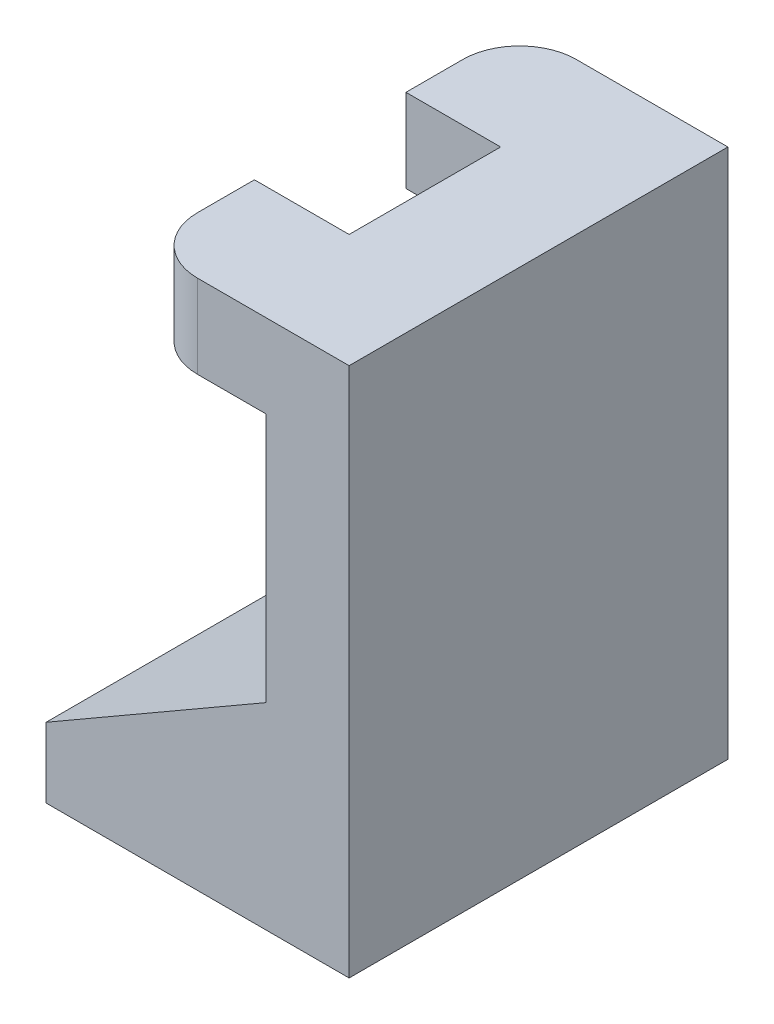
ISO-10303-21;
HEADER;
FILE_DESCRIPTION(('STEP AP214'),'2;1');
FILE_NAME('part.step','',(''),(''),'','','');
FILE_SCHEMA(('AUTOMOTIVE_DESIGN { 1 0 10303 214 1 1 1 1 }'));
ENDSEC;
DATA;
#1=APPLICATION_CONTEXT('core data for automotive mechanical design processes');
#2=APPLICATION_PROTOCOL_DEFINITION('international standard','automotive_design',2000,#1);
#3=PRODUCT_CONTEXT('',#1,'mechanical');
#4=PRODUCT('Part','Part','',(#3));
#5=PRODUCT_RELATED_PRODUCT_CATEGORY('part','',(#4));
#6=PRODUCT_DEFINITION_FORMATION('','',#4);
#7=PRODUCT_DEFINITION_CONTEXT('part definition',#1,'design');
#8=PRODUCT_DEFINITION('design','',#6,#7);
#9=PRODUCT_DEFINITION_SHAPE('','',#8);
#10=(LENGTH_UNIT() NAMED_UNIT(*) SI_UNIT(.MILLI.,.METRE.));
#11=(NAMED_UNIT(*) PLANE_ANGLE_UNIT() SI_UNIT($,.RADIAN.));
#12=(NAMED_UNIT(*) SI_UNIT($,.STERADIAN.) SOLID_ANGLE_UNIT());
#13=UNCERTAINTY_MEASURE_WITH_UNIT(LENGTH_MEASURE(1.E-05),#10,'distance_accuracy_value','');
#14=(GEOMETRIC_REPRESENTATION_CONTEXT(3) GLOBAL_UNCERTAINTY_ASSIGNED_CONTEXT((#13)) GLOBAL_UNIT_ASSIGNED_CONTEXT((#10,
#11,#12)) REPRESENTATION_CONTEXT('',''));
#15=CARTESIAN_POINT('',(0.,0.,0.));
#16=DIRECTION('',(0.,0.,1.));
#17=DIRECTION('',(1.,0.,0.));
#18=AXIS2_PLACEMENT_3D('',#15,#16,#17);
#19=CARTESIAN_POINT('',(0.5,2.8,-2.));
#20=DIRECTION('',(-1.,0.,0.));
#21=DIRECTION('',(0.,-1.,0.));
#22=AXIS2_PLACEMENT_3D('',#19,#20,#21);
#23=PLANE('',#22);
#24=DIRECTION('',(0.,1.,0.));
#25=VECTOR('',#24,1.);
#26=CARTESIAN_POINT('',(0.5,2.36,-0.6));
#27=LINE('',#26,#25);
#28=CARTESIAN_POINT('',(0.5,2.36,-0.6));
#29=VERTEX_POINT('',#28);
#30=CARTESIAN_POINT('',(0.5,2.8,-0.6));
#31=VERTEX_POINT('',#30);
#32=EDGE_CURVE('E181',#29,#31,#27,.T.);
#33=ORIENTED_EDGE('',*,*,#32,.F.);
#34=DIRECTION('',(0.,0.,1.));
#35=VECTOR('',#34,1.);
#36=CARTESIAN_POINT('',(0.5,2.36,-2.));
#37=LINE('',#36,#35);
#38=CARTESIAN_POINT('',(0.5,2.36,-0.3));
#39=VERTEX_POINT('',#38);
#40=EDGE_CURVE('E246',#29,#39,#37,.T.);
#41=ORIENTED_EDGE('',*,*,#40,.T.);
#42=DIRECTION('',(0.,1.,0.));
#43=VECTOR('',#42,1.);
#44=CARTESIAN_POINT('',(0.5,2.36,-0.3));
#45=LINE('',#44,#43);
#46=CARTESIAN_POINT('',(0.5,2.8,-0.3));
#47=VERTEX_POINT('',#46);
#48=EDGE_CURVE('E192',#39,#47,#45,.T.);
#49=ORIENTED_EDGE('',*,*,#48,.T.);
#50=DIRECTION('',(0.,0.,1.));
#51=VECTOR('',#50,1.);
#52=CARTESIAN_POINT('',(0.5,2.8,-2.));
#53=LINE('',#52,#51);
#54=EDGE_CURVE('E255',#31,#47,#53,.T.);
#55=ORIENTED_EDGE('',*,*,#54,.F.);
#56=EDGE_LOOP('',(#33,#41,#49,#55));
#57=FACE_BOUND('',#56,.T.);
#58=ADVANCED_FACE('F44',(#57),#23,.T.);
#59=DIRECTION('',(0.,1.,0.));
#60=VECTOR('',#59,1.);
#61=CARTESIAN_POINT('',(0.5,2.36,-1.4));
#62=LINE('',#61,#60);
#63=CARTESIAN_POINT('',(0.5,2.36,-1.4));
#64=VERTEX_POINT('',#63);
#65=CARTESIAN_POINT('',(0.5,2.8,-1.4));
#66=VERTEX_POINT('',#65);
#67=EDGE_CURVE('E160',#64,#66,#62,.T.);
#68=ORIENTED_EDGE('',*,*,#67,.T.);
#69=CARTESIAN_POINT('',(0.5,2.8,-1.7));
#70=VERTEX_POINT('',#69);
#71=EDGE_CURVE('E253',#70,#66,#53,.T.);
#72=ORIENTED_EDGE('',*,*,#71,.F.);
#73=DIRECTION('',(0.,1.,0.));
#74=VECTOR('',#73,1.);
#75=CARTESIAN_POINT('',(0.5,2.36,-1.7));
#76=LINE('',#75,#74);
#77=CARTESIAN_POINT('',(0.5,2.36,-1.7));
#78=VERTEX_POINT('',#77);
#79=EDGE_CURVE('E189',#78,#70,#76,.T.);
#80=ORIENTED_EDGE('',*,*,#79,.F.);
#81=EDGE_CURVE('E248',#78,#64,#37,.T.);
#82=ORIENTED_EDGE('',*,*,#81,.T.);
#83=EDGE_LOOP('',(#68,#72,#80,#82));
#84=FACE_BOUND('',#83,.T.);
#85=ADVANCED_FACE('F296',(#84),#23,.T.);
#86=CARTESIAN_POINT('',(0.,0.,-2.));
#87=DIRECTION('',(0.,0.,1.));
#88=DIRECTION('',(1.,0.,0.));
#89=AXIS2_PLACEMENT_3D('',#86,#87,#88);
#90=PLANE('',#89);
#91=DIRECTION('',(0.,1.,0.));
#92=VECTOR('',#91,1.);
#93=CARTESIAN_POINT('',(0.8,2.36,-2.));
#94=LINE('',#93,#92);
#95=CARTESIAN_POINT('',(0.8,2.36,-2.));
#96=VERTEX_POINT('',#95);
#97=CARTESIAN_POINT('',(0.8,2.8,-2.));
#98=VERTEX_POINT('',#97);
#99=EDGE_CURVE('E195',#96,#98,#94,.T.);
#100=ORIENTED_EDGE('',*,*,#99,.T.);
#101=DIRECTION('',(-1.,0.,0.));
#102=VECTOR('',#101,1.);
#103=CARTESIAN_POINT('',(1.6,2.8,-2.));
#104=LINE('',#103,#102);
#105=CARTESIAN_POINT('',(1.6,2.8,-2.));
#106=VERTEX_POINT('',#105);
#107=EDGE_CURVE('E214',#106,#98,#104,.T.);
#108=ORIENTED_EDGE('',*,*,#107,.F.);
#109=DIRECTION('',(0.,1.,0.));
#110=VECTOR('',#109,1.);
#111=CARTESIAN_POINT('',(1.6,0.,-2.));
#112=LINE('',#111,#110);
#113=CARTESIAN_POINT('',(1.6,0.,-2.));
#114=VERTEX_POINT('',#113);
#115=EDGE_CURVE('E215',#114,#106,#112,.T.);
#116=ORIENTED_EDGE('',*,*,#115,.F.);
#117=DIRECTION('',(1.,0.,0.));
#118=VECTOR('',#117,1.);
#119=CARTESIAN_POINT('',(0.,0.,-2.));
#120=LINE('',#119,#118);
#121=CARTESIAN_POINT('',(0.,0.,-2.));
#122=VERTEX_POINT('',#121);
#123=EDGE_CURVE('E208',#122,#114,#120,.T.);
#124=ORIENTED_EDGE('',*,*,#123,.F.);
#125=DIRECTION('',(0.,-1.,0.));
#126=VECTOR('',#125,1.);
#127=CARTESIAN_POINT('',(0.,0.,-2.));
#128=LINE('',#127,#126);
#129=CARTESIAN_POINT('',(0.,0.369422221254713,-2.));
#130=VERTEX_POINT('',#129);
#131=EDGE_CURVE('E202',#130,#122,#128,.T.);
#132=ORIENTED_EDGE('',*,*,#131,.F.);
#133=DIRECTION('',(-0.866025403784438,-0.500000000000001,0.));
#134=VECTOR('',#133,1.);
#135=CARTESIAN_POINT('',(0.,0.369422221254713,-2.));
#136=LINE('',#135,#134);
#137=CARTESIAN_POINT('',(1.16,1.03914853351468,-2.));
#138=VERTEX_POINT('',#137);
#139=EDGE_CURVE('E224',#138,#130,#136,.T.);
#140=ORIENTED_EDGE('',*,*,#139,.F.);
#141=DIRECTION('',(0.,-1.,0.));
#142=VECTOR('',#141,1.);
#143=CARTESIAN_POINT('',(1.16,2.36,-2.));
#144=LINE('',#143,#142);
#145=CARTESIAN_POINT('',(1.16,2.36,-2.));
#146=VERTEX_POINT('',#145);
#147=EDGE_CURVE('E219',#146,#138,#144,.T.);
#148=ORIENTED_EDGE('',*,*,#147,.F.);
#149=DIRECTION('',(1.,0.,0.));
#150=VECTOR('',#149,1.);
#151=CARTESIAN_POINT('',(1.16,2.36,-2.));
#152=LINE('',#151,#150);
#153=EDGE_CURVE('E217',#96,#146,#152,.T.);
#154=ORIENTED_EDGE('',*,*,#153,.F.);
#155=EDGE_LOOP('',(#100,#108,#116,#124,#132,#140,#148,#154));
#156=FACE_BOUND('',#155,.T.);
#157=ADVANCED_FACE('F272',(#156),#90,.F.);
#158=CARTESIAN_POINT('',(0.,0.,0.));
#159=DIRECTION('',(0.,0.,1.));
#160=DIRECTION('',(1.,0.,0.));
#161=AXIS2_PLACEMENT_3D('',#158,#159,#160);
#162=PLANE('',#161);
#163=DIRECTION('',(-1.,0.,0.));
#164=VECTOR('',#163,1.);
#165=CARTESIAN_POINT('',(1.6,2.8,0.));
#166=LINE('',#165,#164);
#167=CARTESIAN_POINT('',(1.6,2.8,0.));
#168=VERTEX_POINT('',#167);
#169=CARTESIAN_POINT('',(0.8,2.8,0.));
#170=VERTEX_POINT('',#169);
#171=EDGE_CURVE('E234',#168,#170,#166,.T.);
#172=ORIENTED_EDGE('',*,*,#171,.T.);
#173=DIRECTION('',(0.,1.,0.));
#174=VECTOR('',#173,1.);
#175=CARTESIAN_POINT('',(0.8,2.36,0.));
#176=LINE('',#175,#174);
#177=CARTESIAN_POINT('',(0.8,2.36,0.));
#178=VERTEX_POINT('',#177);
#179=EDGE_CURVE('E200',#178,#170,#176,.T.);
#180=ORIENTED_EDGE('',*,*,#179,.F.);
#181=DIRECTION('',(1.,0.,0.));
#182=VECTOR('',#181,1.);
#183=CARTESIAN_POINT('',(1.16,2.36,0.));
#184=LINE('',#183,#182);
#185=CARTESIAN_POINT('',(1.16,2.36,0.));
#186=VERTEX_POINT('',#185);
#187=EDGE_CURVE('E240',#178,#186,#184,.T.);
#188=ORIENTED_EDGE('',*,*,#187,.T.);
#189=DIRECTION('',(0.,-1.,0.));
#190=VECTOR('',#189,1.);
#191=CARTESIAN_POINT('',(1.16,2.36,0.));
#192=LINE('',#191,#190);
#193=CARTESIAN_POINT('',(1.16,1.03914853351468,0.));
#194=VERTEX_POINT('',#193);
#195=EDGE_CURVE('E239',#186,#194,#192,.T.);
#196=ORIENTED_EDGE('',*,*,#195,.T.);
#197=DIRECTION('',(-0.866025403784438,-0.500000000000001,0.));
#198=VECTOR('',#197,1.);
#199=CARTESIAN_POINT('',(0.,0.369422221254713,0.));
#200=LINE('',#199,#198);
#201=CARTESIAN_POINT('',(0.,0.369422221254713,0.));
#202=VERTEX_POINT('',#201);
#203=EDGE_CURVE('E207',#194,#202,#200,.T.);
#204=ORIENTED_EDGE('',*,*,#203,.T.);
#205=DIRECTION('',(0.,-1.,0.));
#206=VECTOR('',#205,1.);
#207=CARTESIAN_POINT('',(0.,0.,0.));
#208=LINE('',#207,#206);
#209=CARTESIAN_POINT('',(0.,0.,0.));
#210=VERTEX_POINT('',#209);
#211=EDGE_CURVE('E194',#202,#210,#208,.T.);
#212=ORIENTED_EDGE('',*,*,#211,.T.);
#213=DIRECTION('',(1.,0.,0.));
#214=VECTOR('',#213,1.);
#215=CARTESIAN_POINT('',(0.,0.,0.));
#216=LINE('',#215,#214);
#217=CARTESIAN_POINT('',(1.6,0.,0.));
#218=VERTEX_POINT('',#217);
#219=EDGE_CURVE('E226',#210,#218,#216,.T.);
#220=ORIENTED_EDGE('',*,*,#219,.T.);
#221=DIRECTION('',(0.,1.,0.));
#222=VECTOR('',#221,1.);
#223=CARTESIAN_POINT('',(1.6,0.,0.));
#224=LINE('',#223,#222);
#225=EDGE_CURVE('E232',#218,#168,#224,.T.);
#226=ORIENTED_EDGE('',*,*,#225,.T.);
#227=EDGE_LOOP('',(#172,#180,#188,#196,#204,#212,#220,#226));
#228=FACE_BOUND('',#227,.T.);
#229=ADVANCED_FACE('F266',(#228),#162,.T.);
#230=CARTESIAN_POINT('',(0.,0.,-2.));
#231=DIRECTION('',(-1.,0.,0.));
#232=DIRECTION('',(0.,0.,1.));
#233=AXIS2_PLACEMENT_3D('',#230,#231,#232);
#234=PLANE('',#233);
#235=ORIENTED_EDGE('',*,*,#211,.F.);
#236=DIRECTION('',(0.,0.,1.));
#237=VECTOR('',#236,1.);
#238=CARTESIAN_POINT('',(0.,0.369422221254713,-2.));
#239=LINE('',#238,#237);
#240=EDGE_CURVE('E11',#130,#202,#239,.T.);
#241=ORIENTED_EDGE('',*,*,#240,.F.);
#242=ORIENTED_EDGE('',*,*,#131,.T.);
#243=DIRECTION('',(0.,0.,1.));
#244=VECTOR('',#243,1.);
#245=CARTESIAN_POINT('',(0.,0.,-2.));
#246=LINE('',#245,#244);
#247=EDGE_CURVE('E47',#122,#210,#246,.T.);
#248=ORIENTED_EDGE('',*,*,#247,.T.);
#249=EDGE_LOOP('',(#235,#241,#242,#248));
#250=FACE_BOUND('',#249,.T.);
#251=ADVANCED_FACE('F50',(#250),#234,.T.);
#252=CARTESIAN_POINT('',(0.,0.369422221254713,-2.));
#253=DIRECTION('',(-0.500000000000001,0.866025403784438,0.));
#254=DIRECTION('',(-0.866025403784438,-0.500000000000001,0.));
#255=AXIS2_PLACEMENT_3D('',#252,#253,#254);
#256=PLANE('',#255);
#257=CARTESIAN_POINT('',(0.6,0.715832382768489,-1.));
#258=DIRECTION('',(-0.500000000000001,0.866025403784438,0.));
#259=DIRECTION('',(-0.866025403784438,-0.500000000000001,0.));
#260=AXIS2_PLACEMENT_3D('',#257,#258,#259);
#261=ELLIPSE('',#260,0.230940107675851,0.2);
#262=CARTESIAN_POINT('',(0.4,0.600362328930564,-1.));
#263=VERTEX_POINT('',#262);
#264=EDGE_CURVE('E174',#263,#263,#261,.T.);
#265=ORIENTED_EDGE('',*,*,#264,.F.);
#266=EDGE_LOOP('',(#265));
#267=FACE_BOUND('',#266,.T.);
#268=ORIENTED_EDGE('',*,*,#203,.F.);
#269=DIRECTION('',(0.,0.,1.));
#270=VECTOR('',#269,1.);
#271=CARTESIAN_POINT('',(1.16,1.03914853351468,-2.));
#272=LINE('',#271,#270);
#273=EDGE_CURVE('E53',#138,#194,#272,.T.);
#274=ORIENTED_EDGE('',*,*,#273,.F.);
#275=ORIENTED_EDGE('',*,*,#139,.T.);
#276=ORIENTED_EDGE('',*,*,#240,.T.);
#277=EDGE_LOOP('',(#268,#274,#275,#276));
#278=FACE_BOUND('',#277,.T.);
#279=ADVANCED_FACE('F269',(#267,#278),#256,.T.);
#280=CARTESIAN_POINT('',(1.16,2.36,-2.));
#281=DIRECTION('',(-1.,0.,0.));
#282=DIRECTION('',(0.,-1.,0.));
#283=AXIS2_PLACEMENT_3D('',#280,#281,#282);
#284=PLANE('',#283);
#285=ORIENTED_EDGE('',*,*,#195,.F.);
#286=DIRECTION('',(0.,0.,1.));
#287=VECTOR('',#286,1.);
#288=CARTESIAN_POINT('',(1.16,2.36,-2.));
#289=LINE('',#288,#287);
#290=EDGE_CURVE('E242',#146,#186,#289,.T.);
#291=ORIENTED_EDGE('',*,*,#290,.F.);
#292=ORIENTED_EDGE('',*,*,#147,.T.);
#293=ORIENTED_EDGE('',*,*,#273,.T.);
#294=EDGE_LOOP('',(#285,#291,#292,#293));
#295=FACE_BOUND('',#294,.T.);
#296=ADVANCED_FACE('F294',(#295),#284,.T.);
#297=CARTESIAN_POINT('',(1.16,2.36,-2.));
#298=DIRECTION('',(0.,-1.,0.));
#299=DIRECTION('',(0.,0.,-1.));
#300=AXIS2_PLACEMENT_3D('',#297,#298,#299);
#301=PLANE('',#300);
#302=DIRECTION('',(1.,0.,0.));
#303=VECTOR('',#302,1.);
#304=CARTESIAN_POINT('',(0.5,2.36,-0.6));
#305=LINE('',#304,#303);
#306=CARTESIAN_POINT('',(1.,2.36,-0.6));
#307=VERTEX_POINT('',#306);
#308=EDGE_CURVE('E158',#29,#307,#305,.T.);
#309=ORIENTED_EDGE('',*,*,#308,.T.);
#310=DIRECTION('',(0.,0.,-1.));
#311=VECTOR('',#310,1.);
#312=CARTESIAN_POINT('',(1.,2.36,-0.6));
#313=LINE('',#312,#311);
#314=CARTESIAN_POINT('',(1.,2.36,-1.4));
#315=VERTEX_POINT('',#314);
#316=EDGE_CURVE('E151',#307,#315,#313,.T.);
#317=ORIENTED_EDGE('',*,*,#316,.T.);
#318=DIRECTION('',(-1.,0.,0.));
#319=VECTOR('',#318,1.);
#320=CARTESIAN_POINT('',(1.,2.36,-1.4));
#321=LINE('',#320,#319);
#322=EDGE_CURVE('E161',#315,#64,#321,.T.);
#323=ORIENTED_EDGE('',*,*,#322,.T.);
#324=ORIENTED_EDGE('',*,*,#81,.F.);
#325=CARTESIAN_POINT('',(0.8,2.36,-1.7));
#326=DIRECTION('',(0.,-1.,0.));
#327=DIRECTION('',(0.,0.,1.));
#328=AXIS2_PLACEMENT_3D('',#325,#326,#327);
#329=CIRCLE('',#328,0.3);
#330=EDGE_CURVE('E188',#78,#96,#329,.T.);
#331=ORIENTED_EDGE('',*,*,#330,.T.);
#332=ORIENTED_EDGE('',*,*,#153,.T.);
#333=ORIENTED_EDGE('',*,*,#290,.T.);
#334=ORIENTED_EDGE('',*,*,#187,.F.);
#335=CARTESIAN_POINT('',(0.8,2.36,-0.3));
#336=DIRECTION('',(0.,-1.,0.));
#337=DIRECTION('',(0.,0.,1.));
#338=AXIS2_PLACEMENT_3D('',#335,#336,#337);
#339=CIRCLE('',#338,0.3);
#340=EDGE_CURVE('E198',#178,#39,#339,.T.);
#341=ORIENTED_EDGE('',*,*,#340,.T.);
#342=ORIENTED_EDGE('',*,*,#40,.F.);
#343=EDGE_LOOP('',(#309,#317,#323,#324,#331,#332,#333,#334,#341,#342));
#344=FACE_BOUND('',#343,.T.);
#345=ADVANCED_FACE('F169',(#344),#301,.T.);
#346=CARTESIAN_POINT('',(1.6,2.8,-2.));
#347=DIRECTION('',(0.,1.,0.));
#348=DIRECTION('',(0.,0.,1.));
#349=AXIS2_PLACEMENT_3D('',#346,#347,#348);
#350=PLANE('',#349);
#351=DIRECTION('',(1.,0.,0.));
#352=VECTOR('',#351,1.);
#353=CARTESIAN_POINT('',(0.5,2.8,-0.6));
#354=LINE('',#353,#352);
#355=CARTESIAN_POINT('',(1.,2.8,-0.6));
#356=VERTEX_POINT('',#355);
#357=EDGE_CURVE('E65',#31,#356,#354,.T.);
#358=ORIENTED_EDGE('',*,*,#357,.F.);
#359=ORIENTED_EDGE('',*,*,#54,.T.);
#360=CARTESIAN_POINT('',(0.8,2.8,-0.3));
#361=DIRECTION('',(0.,-1.,0.));
#362=DIRECTION('',(0.,0.,1.));
#363=AXIS2_PLACEMENT_3D('',#360,#361,#362);
#364=CIRCLE('',#363,0.3);
#365=EDGE_CURVE('E185',#170,#47,#364,.T.);
#366=ORIENTED_EDGE('',*,*,#365,.F.);
#367=ORIENTED_EDGE('',*,*,#171,.F.);
#368=DIRECTION('',(0.,0.,1.));
#369=VECTOR('',#368,1.);
#370=CARTESIAN_POINT('',(1.6,2.8,-2.));
#371=LINE('',#370,#369);
#372=EDGE_CURVE('E254',#106,#168,#371,.T.);
#373=ORIENTED_EDGE('',*,*,#372,.F.);
#374=ORIENTED_EDGE('',*,*,#107,.T.);
#375=CARTESIAN_POINT('',(0.8,2.8,-1.7));
#376=DIRECTION('',(0.,-1.,0.));
#377=DIRECTION('',(0.,0.,1.));
#378=AXIS2_PLACEMENT_3D('',#375,#376,#377);
#379=CIRCLE('',#378,0.3);
#380=EDGE_CURVE('E66',#70,#98,#379,.T.);
#381=ORIENTED_EDGE('',*,*,#380,.F.);
#382=ORIENTED_EDGE('',*,*,#71,.T.);
#383=DIRECTION('',(-1.,0.,0.));
#384=VECTOR('',#383,1.);
#385=CARTESIAN_POINT('',(1.,2.8,-1.4));
#386=LINE('',#385,#384);
#387=CARTESIAN_POINT('',(1.,2.8,-1.4));
#388=VERTEX_POINT('',#387);
#389=EDGE_CURVE('E173',#388,#66,#386,.T.);
#390=ORIENTED_EDGE('',*,*,#389,.F.);
#391=DIRECTION('',(0.,0.,-1.));
#392=VECTOR('',#391,1.);
#393=CARTESIAN_POINT('',(1.,2.8,-1.));
#394=LINE('',#393,#392);
#395=EDGE_CURVE('E152',#356,#388,#394,.T.);
#396=ORIENTED_EDGE('',*,*,#395,.F.);
#397=EDGE_LOOP('',(#358,#359,#366,#367,#373,#374,#381,#382,#390,#396));
#398=FACE_BOUND('',#397,.T.);
#399=ADVANCED_FACE('F284',(#398),#350,.T.);
#400=CARTESIAN_POINT('',(1.6,0.,-2.));
#401=DIRECTION('',(1.,0.,0.));
#402=DIRECTION('',(0.,0.,-1.));
#403=AXIS2_PLACEMENT_3D('',#400,#401,#402);
#404=PLANE('',#403);
#405=ORIENTED_EDGE('',*,*,#225,.F.);
#406=DIRECTION('',(0.,0.,1.));
#407=VECTOR('',#406,1.);
#408=CARTESIAN_POINT('',(1.6,0.,-2.));
#409=LINE('',#408,#407);
#410=EDGE_CURVE('E258',#114,#218,#409,.T.);
#411=ORIENTED_EDGE('',*,*,#410,.F.);
#412=ORIENTED_EDGE('',*,*,#115,.T.);
#413=ORIENTED_EDGE('',*,*,#372,.T.);
#414=EDGE_LOOP('',(#405,#411,#412,#413));
#415=FACE_BOUND('',#414,.T.);
#416=ADVANCED_FACE('F279',(#415),#404,.T.);
#417=CARTESIAN_POINT('',(0.,0.,-2.));
#418=DIRECTION('',(0.,-1.,0.));
#419=DIRECTION('',(0.,0.,-1.));
#420=AXIS2_PLACEMENT_3D('',#417,#418,#419);
#421=PLANE('',#420);
#422=CARTESIAN_POINT('',(0.6,0.,-1.));
#423=DIRECTION('',(0.,-1.,0.));
#424=DIRECTION('',(0.,0.,-1.));
#425=AXIS2_PLACEMENT_3D('',#422,#423,#424);
#426=CIRCLE('',#425,0.2);
#427=CARTESIAN_POINT('',(0.6,0.,-1.2));
#428=VERTEX_POINT('',#427);
#429=EDGE_CURVE('E328',#428,#428,#426,.T.);
#430=ORIENTED_EDGE('',*,*,#429,.F.);
#431=EDGE_LOOP('',(#430));
#432=FACE_BOUND('',#431,.T.);
#433=ORIENTED_EDGE('',*,*,#219,.F.);
#434=ORIENTED_EDGE('',*,*,#247,.F.);
#435=ORIENTED_EDGE('',*,*,#123,.T.);
#436=ORIENTED_EDGE('',*,*,#410,.T.);
#437=EDGE_LOOP('',(#433,#434,#435,#436));
#438=FACE_BOUND('',#437,.T.);
#439=ADVANCED_FACE('F262',(#432,#438),#421,.T.);
#440=CARTESIAN_POINT('',(0.8,2.36,-0.3));
#441=DIRECTION('',(0.,1.,0.));
#442=DIRECTION('',(0.,0.,1.));
#443=AXIS2_PLACEMENT_3D('',#440,#441,#442);
#444=CYLINDRICAL_SURFACE('',#443,0.3);
#445=ORIENTED_EDGE('',*,*,#365,.T.);
#446=ORIENTED_EDGE('',*,*,#48,.F.);
#447=ORIENTED_EDGE('',*,*,#340,.F.);
#448=ORIENTED_EDGE('',*,*,#179,.T.);
#449=EDGE_LOOP('',(#445,#446,#447,#448));
#450=FACE_BOUND('',#449,.T.);
#451=ADVANCED_FACE('F288',(#450),#444,.T.);
#452=CARTESIAN_POINT('',(0.8,2.36,-1.7));
#453=DIRECTION('',(0.,1.,0.));
#454=DIRECTION('',(0.,0.,1.));
#455=AXIS2_PLACEMENT_3D('',#452,#453,#454);
#456=CYLINDRICAL_SURFACE('',#455,0.3);
#457=ORIENTED_EDGE('',*,*,#380,.T.);
#458=ORIENTED_EDGE('',*,*,#99,.F.);
#459=ORIENTED_EDGE('',*,*,#330,.F.);
#460=ORIENTED_EDGE('',*,*,#79,.T.);
#461=EDGE_LOOP('',(#457,#458,#459,#460));
#462=FACE_BOUND('',#461,.T.);
#463=ADVANCED_FACE('F299',(#462),#456,.T.);
#464=CARTESIAN_POINT('',(0.5,2.36,-0.6));
#465=DIRECTION('',(0.,0.,1.));
#466=DIRECTION('',(1.,0.,0.));
#467=AXIS2_PLACEMENT_3D('',#464,#465,#466);
#468=PLANE('',#467);
#469=ORIENTED_EDGE('',*,*,#357,.T.);
#470=DIRECTION('',(0.,1.,0.));
#471=VECTOR('',#470,1.);
#472=CARTESIAN_POINT('',(1.,2.36,-0.6));
#473=LINE('',#472,#471);
#474=EDGE_CURVE('E176',#307,#356,#473,.T.);
#475=ORIENTED_EDGE('',*,*,#474,.F.);
#476=ORIENTED_EDGE('',*,*,#308,.F.);
#477=ORIENTED_EDGE('',*,*,#32,.T.);
#478=EDGE_LOOP('',(#469,#475,#476,#477));
#479=FACE_BOUND('',#478,.T.);
#480=ADVANCED_FACE('F302',(#479),#468,.F.);
#481=CARTESIAN_POINT('',(1.,2.36,-1.4));
#482=DIRECTION('',(0.,0.,-1.));
#483=DIRECTION('',(-1.,0.,0.));
#484=AXIS2_PLACEMENT_3D('',#481,#482,#483);
#485=PLANE('',#484);
#486=ORIENTED_EDGE('',*,*,#389,.T.);
#487=ORIENTED_EDGE('',*,*,#67,.F.);
#488=ORIENTED_EDGE('',*,*,#322,.F.);
#489=DIRECTION('',(0.,1.,0.));
#490=VECTOR('',#489,1.);
#491=CARTESIAN_POINT('',(1.,2.36,-1.4));
#492=LINE('',#491,#490);
#493=EDGE_CURVE('E150',#315,#388,#492,.T.);
#494=ORIENTED_EDGE('',*,*,#493,.T.);
#495=EDGE_LOOP('',(#486,#487,#488,#494));
#496=FACE_BOUND('',#495,.T.);
#497=ADVANCED_FACE('F165',(#496),#485,.F.);
#498=CARTESIAN_POINT('',(1.,2.36,-1.));
#499=DIRECTION('',(1.,0.,0.));
#500=DIRECTION('',(0.,0.,-1.));
#501=AXIS2_PLACEMENT_3D('',#498,#499,#500);
#502=PLANE('',#501);
#503=ORIENTED_EDGE('',*,*,#395,.T.);
#504=ORIENTED_EDGE('',*,*,#493,.F.);
#505=ORIENTED_EDGE('',*,*,#316,.F.);
#506=ORIENTED_EDGE('',*,*,#474,.T.);
#507=EDGE_LOOP('',(#503,#504,#505,#506));
#508=FACE_BOUND('',#507,.T.);
#509=ADVANCED_FACE('F149',(#508),#502,.F.);
#510=CARTESIAN_POINT('',(0.6,1.,-1.));
#511=DIRECTION('',(0.,-1.,0.));
#512=DIRECTION('',(0.,0.,-1.));
#513=AXIS2_PLACEMENT_3D('',#510,#511,#512);
#514=CYLINDRICAL_SURFACE('',#513,0.2);
#515=ORIENTED_EDGE('',*,*,#264,.T.);
#516=EDGE_LOOP('',(#515));
#517=FACE_BOUND('',#516,.T.);
#518=ORIENTED_EDGE('',*,*,#429,.T.);
#519=EDGE_LOOP('',(#518));
#520=FACE_BOUND('',#519,.T.);
#521=ADVANCED_FACE('F331',(#517,#520),#514,.F.);
#522=CLOSED_SHELL('',(#58,#85,#157,#229,#251,#279,#296,#345,#399,#416,#439,#451,#463,#480,#497,
#509,#521));
#523=MANIFOLD_SOLID_BREP('B2',#522);
#524=ADVANCED_BREP_SHAPE_REPRESENTATION('',(#18,#523),#14);
#525=SHAPE_DEFINITION_REPRESENTATION(#9,#524);
ENDSEC;
END-ISO-10303-21;
